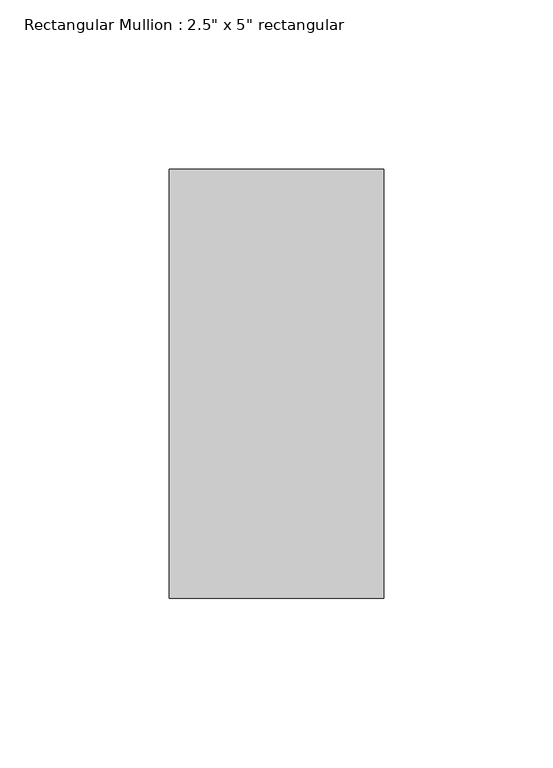
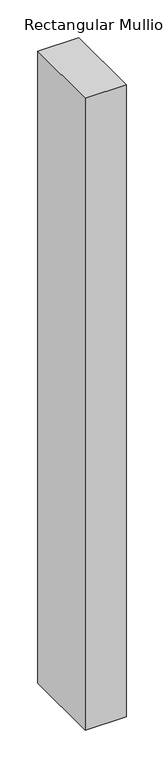
"""IFC4 building model written with IfcOpenShell, lengths in millimetres: member geometry."""

from ifc_helpers import new_model, si_unit, frame, origin, place, context, project, spatial, polyline, outline, extrude, source, transform, mapped, element, save


def member_79ceace6(model_context):
    return source(origin(), model_context, "Body", "SweptSolid", [
        extrude(outline(polyline([(0.0, 63.5), (0.0, -63.5), (-63.5, -63.5), (-63.5, 63.5), (0.0, 63.5)])), frame((0.0, 0.0, -1028.7), z_axis=(0.0, 0.0, 1.0), x_axis=(1.0, 0.0, 0.0)), (0.0, 0.0, 1.0), 1028.7),
    ])


if __name__ == "__main__":
    model = new_model("IFC4")
    model_context = context("Model", 3, world=origin())
    ifc_project = project(units=[si_unit("LENGTHUNIT", "METRE", prefix="MILLI")], contexts=[model_context])
    site = spatial("IfcSite", under=ifc_project)
    building = spatial("IfcBuilding", under=site)
    placement = place(None, origin())
    member_shape = member_79ceace6(model_context)
    element("IfcMember", 1, ObjectType="Rectangular Mullion : 2.5\" x 5\" rectangular", at=placement, inside=building, context=model_context, shape_type="MappedRepresentation", body=[
        mapped(member_shape, transform((0.0, 0.0, 0.0), x_axis=(1.0, 0.0, 0.0), y_axis=(0.0, 1.0, 0.0), z_axis=(0.0, 0.0, 1.0))),
    ])
    save(model, "model.ifc")

# Revit data of these elements
# Type "Rectangular Mullion : 2.5\" x 5\" rectangular"
#   built-in parameter 1007304 = 0.416667 (stored number, unit not read)
#   built-in parameter 1007301 = 0.104167 (stored number, unit not read)
#   built-in parameter 1007300 = 0.104167 (stored number, unit not read)
# Element 1 (IfcMember, "Rectangular Mullion : 2.5\" x 5\" rectangular")
#   Materials on its faces: "Aluminum"
# Materials
#   "Aluminum": class "Metal", colour RGB 247 247 247, transparency 0, Description = "Aluminum 6061", Cost = 0
